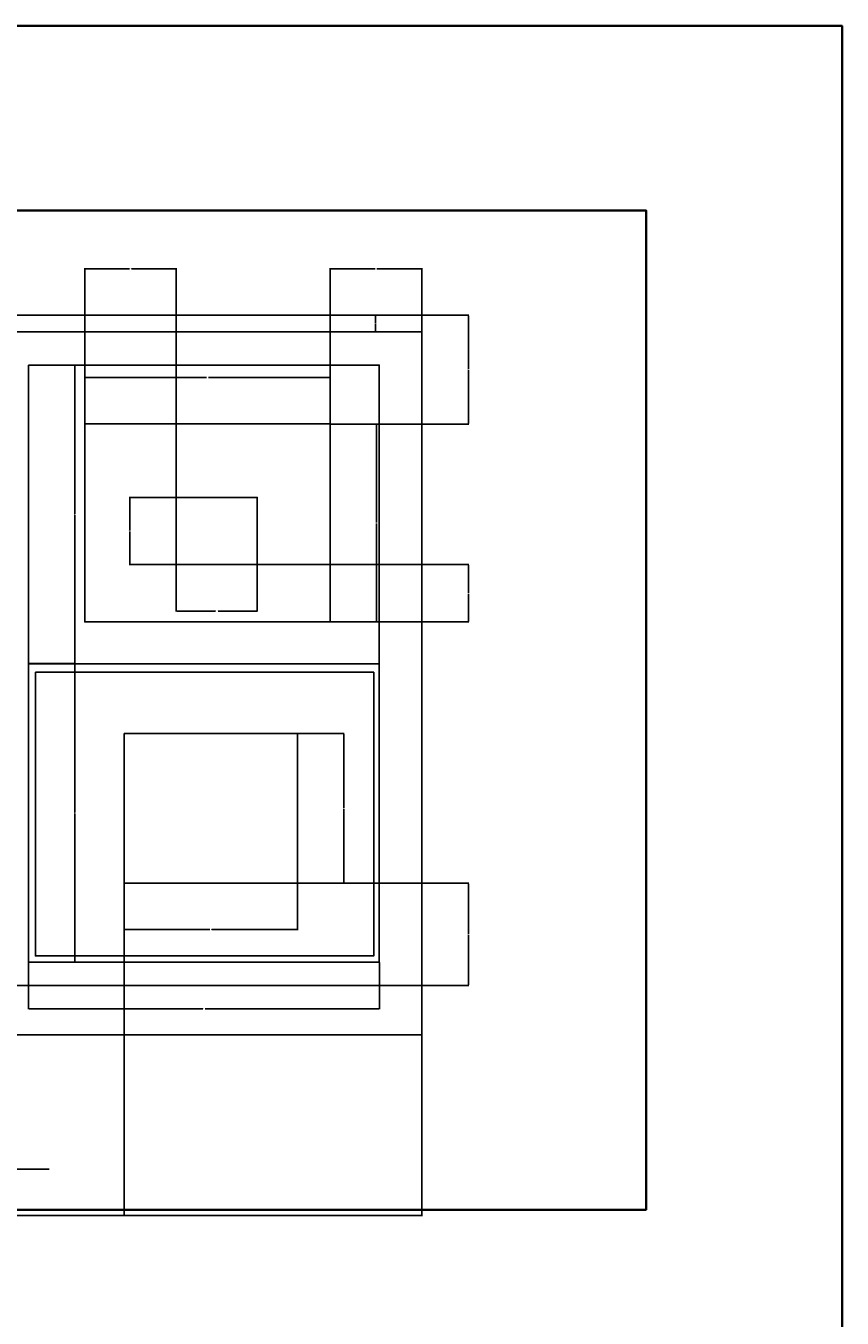
# Model space of a CAD drawing. Units: inches. Extents: x 1976 to 2558, y -977 to 2909.
# Tile 8 of 8: x 2262 to 2558, y 2441 to 2909. Entities that reach past the tile are written whole.
import ezdxf

# ---------------------------------------------------------------- set-up
doc = ezdxf.new("R2010")
doc.units = ezdxf.units.IN
for name, color, linetype, lineweight in [('A-ANNO-DIMS', 2, 'Continuous', 18), ('A-ANNO-TEXT', 7, 'Continuous', 25), ('A-ANNO-TTLB', 7, 'Continuous', 35), ('A-ELEV', 7, 'Continuous', 25)]:
    doc.layers.add(name, color=color, linetype=linetype, lineweight=lineweight)
doc.styles.get("Standard").update_dxf_attribs({"font": 'arial.ttf'})
doc.dimstyles.get("Standard").update_dxf_attribs({"dimtxt": 0.18, "dimasz": 0.18, "dimexe": 0.18, "dimexo": 0.0625, "dimgap": 0.09, "dimtad": 0, "dimtih": 1, "dimtoh": 1, "dimdec": 4, "dimzin": 0, "dimdsep": 46, "dimtxsty": 'Standard', "dimcen": 0.09, "dimadec": 0, "dimazin": 0, "dimtfac": 1, "dimtdec": 4, "dimtofl": 0, "dimtmove": 0, "dimatfit": 3, "dimfxl": 1, "dimtolj": 1, "dimtzin": 0, "dimarcsym": 0})

# ---------------------------------------------------------------- blocks, each defined once
blk = doc.blocks.new('*D51')
at = {"layer": 'A-ANNO-DIMS', "color": 0, "lineweight": -2, "transparency": 16777216}
for p, q in [((2089.7, 2681.2), (2089.7, 2477.53)), ((2405.44, 2543.2), (2405.44, 2477.53)), ((2089.88, 2477.71), (2247.1, 2477.71)), ((2405.26, 2477.71), (2248.03, 2477.71))]:
    blk.add_line(p, q, dxfattribs=at)
at = {"layer": 'A-ANNO-DIMS', "color": 0, "transparency": 16777216}
for points in [[(2089.88, 2477.74), (2089.88, 2477.68), (2089.7, 2477.71)], [(2405.26, 2477.74), (2405.26, 2477.68), (2405.44, 2477.71)]]:
    blk.add_solid(points, dxfattribs=at)
at = {"layer": 'Defpoints', "color": 0, "transparency": 16777216}
for p in [(2089.7, 2681.26), (2405.44, 2543.26), (2405.44, 2477.71)]:
    blk.add_point(p, dxfattribs=at)
at = {"layer": 'A-ANNO-DIMS', "color": 0, "transparency": 16777216, "insert": (2247.57, 2477.71), "char_height": 0.18, "attachment_point": 5}
blk.add_mtext('\\A1;315.74', dxfattribs=at)
blk = doc.blocks.new('*D63')
at = {"layer": 'A-ANNO-DIMS', "color": 0, "lineweight": -2, "transparency": 16777216}
for p, q in [((2372.2, 2764.9), (2389.17, 2764.9)), ((2388.99, 2764.72), (2388.99, 2729.2)), ((2388.99, 2693.31), (2388.99, 2728.83)), ((2372.2, 2693.13), (2389.17, 2693.13))]:
    blk.add_line(p, q, dxfattribs=at)
at = {"layer": 'A-ANNO-DIMS', "color": 0, "transparency": 16777216}
for points in [[(2388.96, 2764.72), (2389.02, 2764.72), (2388.99, 2764.9)], [(2388.96, 2693.31), (2389.02, 2693.31), (2388.99, 2693.13)]]:
    blk.add_solid(points, dxfattribs=at)
at = {"layer": 'Defpoints', "color": 0, "transparency": 16777216}
for p in [(2372.14, 2764.9), (2372.14, 2693.13), (2388.99, 2693.13)]:
    blk.add_point(p, dxfattribs=at)
at = {"layer": 'A-ANNO-DIMS', "color": 0, "transparency": 16777216, "insert": (2388.99, 2729.02), "char_height": 0.18, "attachment_point": 5}
blk.add_mtext('\\A1;71.77', dxfattribs=at)
blk = doc.blocks.new('*D64')
at = {"layer": 'A-ANNO-DIMS', "color": 0, "lineweight": -2, "transparency": 16777216}
for p, q in [((2283.12, 2764.97), (2283.12, 2781.93)), ((2283.3, 2781.75), (2327.23, 2781.75)), ((2371.96, 2781.75), (2328.02, 2781.75)), ((2372.14, 2764.97), (2372.14, 2781.93))]:
    blk.add_line(p, q, dxfattribs=at)
at = {"layer": 'A-ANNO-DIMS', "color": 0, "transparency": 16777216}
for points in [[(2283.3, 2781.78), (2283.3, 2781.72), (2283.12, 2781.75)], [(2371.96, 2781.78), (2371.96, 2781.72), (2372.14, 2781.75)]]:
    blk.add_solid(points, dxfattribs=at)
at = {"layer": 'Defpoints', "color": 0, "transparency": 16777216}
for p in [(2372.14, 2781.75), (2283.12, 2764.9), (2372.14, 2764.9)]:
    blk.add_point(p, dxfattribs=at)
at = {"layer": 'A-ANNO-DIMS', "color": 0, "transparency": 16777216, "insert": (2327.63, 2781.75), "char_height": 0.18, "attachment_point": 5}
blk.add_mtext('\\A1;89.02', dxfattribs=at)
blk = doc.blocks.new('*D65')
at = {"layer": 'A-ANNO-DIMS', "color": 0, "lineweight": -2, "transparency": 16777216}
for p, q in [((2297.4, 2598.25), (2297.4, 2581.28)), ((2360.24, 2598.25), (2360.24, 2581.28)), ((2297.58, 2581.46), (2328.43, 2581.46)), ((2360.06, 2581.46), (2329.21, 2581.46))]:
    blk.add_line(p, q, dxfattribs=at)
at = {"layer": 'A-ANNO-DIMS', "color": 0, "transparency": 16777216}
for points in [[(2297.58, 2581.49), (2297.58, 2581.43), (2297.4, 2581.46)], [(2360.06, 2581.49), (2360.06, 2581.43), (2360.24, 2581.46)]]:
    blk.add_solid(points, dxfattribs=at)
at = {"layer": 'Defpoints', "color": 0, "transparency": 16777216}
for p in [(2297.4, 2598.31), (2360.24, 2598.31), (2297.4, 2581.46)]:
    blk.add_point(p, dxfattribs=at)
at = {"layer": 'A-ANNO-DIMS', "color": 0, "transparency": 16777216, "insert": (2328.82, 2581.46), "char_height": 0.18, "attachment_point": 5}
blk.add_mtext('\\A1;62.84', dxfattribs=at)
blk = doc.blocks.new('*D66')
at = {"layer": 'A-ANNO-DIMS', "color": 0, "lineweight": -2, "transparency": 16777216}
for p, q in [((2360.3, 2652.57), (2377.27, 2652.57)), ((2377.09, 2652.39), (2377.09, 2625.62)), ((2377.09, 2598.49), (2377.09, 2625.26)), ((2360.3, 2598.31), (2377.27, 2598.31))]:
    blk.add_line(p, q, dxfattribs=at)
at = {"layer": 'A-ANNO-DIMS', "color": 0, "transparency": 16777216}
for points in [[(2377.06, 2652.39), (2377.12, 2652.39), (2377.09, 2652.57)], [(2377.06, 2598.49), (2377.12, 2598.49), (2377.09, 2598.31)]]:
    blk.add_solid(points, dxfattribs=at)
at = {"layer": 'Defpoints', "color": 0, "transparency": 16777216}
for p in [(2360.24, 2652.57), (2360.24, 2598.31), (2377.09, 2598.31)]:
    blk.add_point(p, dxfattribs=at)
at = {"layer": 'A-ANNO-DIMS', "color": 0, "transparency": 16777216, "insert": (2377.09, 2625.44), "char_height": 0.18, "attachment_point": 5}
blk.add_mtext('\\A1;54.26', dxfattribs=at)
blk = doc.blocks.new('*D67')
at = {"layer": 'A-ANNO-DIMS', "color": 0, "lineweight": -2, "transparency": 16777216}
for p, q in [((2297.4, 2598.25), (2297.4, 2477.53)), ((2249.44, 2561.2), (2249.44, 2477.53)), ((2249.62, 2477.71), (2273.02, 2477.71)), ((2297.22, 2477.71), (2273.82, 2477.71))]:
    blk.add_line(p, q, dxfattribs=at)
at = {"layer": 'A-ANNO-DIMS', "color": 0, "transparency": 16777216}
for points in [[(2249.62, 2477.74), (2249.62, 2477.68), (2249.44, 2477.71)], [(2297.22, 2477.74), (2297.22, 2477.68), (2297.4, 2477.71)]]:
    blk.add_solid(points, dxfattribs=at)
at = {"layer": 'Defpoints', "color": 0, "transparency": 16777216}
for p in [(2297.4, 2598.31), (2249.44, 2561.26), (2249.44, 2477.71)]:
    blk.add_point(p, dxfattribs=at)
at = {"layer": 'A-ANNO-DIMS', "color": 0, "transparency": 16777216, "insert": (2273.42, 2477.71), "char_height": 0.18, "attachment_point": 5}
blk.add_mtext('\\A1;47.96', dxfattribs=at)
blk = doc.blocks.new('*D68')
at = {"layer": 'A-ANNO-DIMS', "color": 0, "lineweight": -2, "transparency": 16777216}
for p, q in [((2372.14, 2764.97), (2372.14, 2821.39)), ((2372.32, 2821.21), (2388.46, 2821.21)), ((2405.26, 2821.21), (2389.11, 2821.21)), ((2405.44, 2804.43), (2405.44, 2821.39))]:
    blk.add_line(p, q, dxfattribs=at)
at = {"layer": 'A-ANNO-DIMS', "color": 0, "transparency": 16777216}
for points in [[(2372.32, 2821.24), (2372.32, 2821.18), (2372.14, 2821.21)], [(2405.26, 2821.24), (2405.26, 2821.18), (2405.44, 2821.21)]]:
    blk.add_solid(points, dxfattribs=at)
at = {"layer": 'Defpoints', "color": 0, "transparency": 16777216}
for p in [(2405.44, 2821.21), (2405.44, 2804.36), (2372.14, 2764.9)]:
    blk.add_point(p, dxfattribs=at)
at = {"layer": 'A-ANNO-DIMS', "color": 0, "transparency": 16777216, "insert": (2388.79, 2821.21), "char_height": 0.18, "attachment_point": 5}
blk.add_mtext('\\A1;33.3', dxfattribs=at)
blk = doc.blocks.new('*D69')
at = {"layer": 'A-ANNO-DIMS', "color": 0, "lineweight": -2, "transparency": 16777216}
for p, q in [((2405.5, 2804.36), (2422.47, 2804.36)), ((2422.29, 2804.18), (2422.29, 2784.81)), ((2422.29, 2765.08), (2422.29, 2784.45)), ((2372.2, 2764.9), (2422.47, 2764.9))]:
    blk.add_line(p, q, dxfattribs=at)
at = {"layer": 'A-ANNO-DIMS', "color": 0, "transparency": 16777216}
for points in [[(2422.26, 2804.18), (2422.32, 2804.18), (2422.29, 2804.36)], [(2422.26, 2765.08), (2422.32, 2765.08), (2422.29, 2764.9)]]:
    blk.add_solid(points, dxfattribs=at)
at = {"layer": 'Defpoints', "color": 0, "transparency": 16777216}
for p in [(2405.44, 2804.36), (2422.29, 2804.36), (2372.14, 2764.9)]:
    blk.add_point(p, dxfattribs=at)
at = {"layer": 'A-ANNO-DIMS', "color": 0, "transparency": 16777216, "insert": (2422.29, 2784.63), "char_height": 0.18, "attachment_point": 5}
blk.add_mtext('\\A1;39.46', dxfattribs=at)
blk = doc.blocks.new('*D70')
at = {"layer": 'A-ANNO-DIMS', "color": 0, "lineweight": -2, "transparency": 16777216}
for p, q in [((2360.3, 2598.31), (2422.47, 2598.31)), ((2422.29, 2598.13), (2422.29, 2579.97)), ((2422.29, 2561.44), (2422.29, 2579.6)), ((2405.5, 2561.26), (2422.47, 2561.26))]:
    blk.add_line(p, q, dxfattribs=at)
at = {"layer": 'A-ANNO-DIMS', "color": 0, "transparency": 16777216}
for points in [[(2422.26, 2598.13), (2422.32, 2598.13), (2422.29, 2598.31)], [(2422.26, 2561.44), (2422.32, 2561.44), (2422.29, 2561.26)]]:
    blk.add_solid(points, dxfattribs=at)
at = {"layer": 'Defpoints', "color": 0, "transparency": 16777216}
for p in [(2360.24, 2598.31), (2405.44, 2561.26), (2422.29, 2561.26)]:
    blk.add_point(p, dxfattribs=at)
at = {"layer": 'A-ANNO-DIMS', "color": 0, "transparency": 16777216, "insert": (2422.29, 2579.79), "char_height": 0.18, "attachment_point": 5}
blk.add_mtext('\\A1;37.05', dxfattribs=at)
blk = doc.blocks.new('*D80')
at = {"layer": 'A-ANNO-DIMS', "color": 0, "lineweight": -2, "transparency": 16777216}
for p, q in [((2316.29, 2713.84), (2316.29, 2696.87)), ((2345.68, 2713.84), (2345.68, 2696.87)), ((2316.47, 2697.05), (2330.52, 2697.05)), ((2345.5, 2697.05), (2331.45, 2697.05))]:
    blk.add_line(p, q, dxfattribs=at)
at = {"layer": 'A-ANNO-DIMS', "color": 0, "transparency": 16777216}
for points in [[(2316.47, 2697.08), (2316.47, 2697.02), (2316.29, 2697.05)], [(2345.5, 2697.08), (2345.5, 2697.02), (2345.68, 2697.05)]]:
    blk.add_solid(points, dxfattribs=at)
at = {"layer": 'Defpoints', "color": 0, "transparency": 16777216}
for p in [(2316.29, 2713.9), (2345.68, 2713.9), (2316.29, 2697.05)]:
    blk.add_point(p, dxfattribs=at)
at = {"layer": 'A-ANNO-DIMS', "color": 0, "transparency": 16777216, "insert": (2330.99, 2697.05), "char_height": 0.18, "attachment_point": 5}
blk.add_mtext('\\A1;29.394', dxfattribs=at)
blk = doc.blocks.new('*D81')
at = {"layer": 'A-ANNO-DIMS', "color": 0, "lineweight": -2, "transparency": 16777216}
for p, q in [((2316.23, 2738.25), (2299.26, 2738.25)), ((2299.44, 2738.07), (2299.44, 2726.26)), ((2299.44, 2714.08), (2299.44, 2725.9)), ((2316.23, 2713.9), (2299.26, 2713.9))]:
    blk.add_line(p, q, dxfattribs=at)
at = {"layer": 'A-ANNO-DIMS', "color": 0, "transparency": 16777216}
for points in [[(2299.41, 2738.07), (2299.47, 2738.07), (2299.44, 2738.25)], [(2299.41, 2714.08), (2299.47, 2714.08), (2299.44, 2713.9)]]:
    blk.add_solid(points, dxfattribs=at)
at = {"layer": 'Defpoints', "color": 0, "transparency": 16777216}
for p in [(2299.44, 2738.25), (2316.29, 2738.25), (2316.29, 2713.9)]:
    blk.add_point(p, dxfattribs=at)
at = {"layer": 'A-ANNO-DIMS', "color": 0, "transparency": 16777216, "insert": (2299.44, 2726.08), "char_height": 0.18, "attachment_point": 5}
blk.add_mtext('\\A1;24.345', dxfattribs=at)
blk = doc.blocks.new('*D82')
at = {"layer": 'A-ANNO-DIMS', "color": 0, "lineweight": -2, "transparency": 16777216}
for p, q in [((2405.38, 2804.36), (2388.41, 2804.36)), ((2388.59, 2804.18), (2388.59, 2801.54)), ((2388.59, 2798.54), (2388.59, 2801.18)), ((2405.38, 2798.36), (2388.41, 2798.36))]:
    blk.add_line(p, q, dxfattribs=at)
at = {"layer": 'A-ANNO-DIMS', "color": 0, "transparency": 16777216}
for points in [[(2388.56, 2804.18), (2388.62, 2804.18), (2388.59, 2804.36)], [(2388.56, 2798.54), (2388.62, 2798.54), (2388.59, 2798.36)]]:
    blk.add_solid(points, dxfattribs=at)
at = {"layer": 'Defpoints', "color": 0, "transparency": 16777216}
for p in [(2388.59, 2804.36), (2405.44, 2804.36), (2405.44, 2798.36)]:
    blk.add_point(p, dxfattribs=at)
at = {"layer": 'A-ANNO-DIMS', "color": 0, "transparency": 16777216, "insert": (2388.59, 2801.36), "char_height": 0.18, "attachment_point": 5}
blk.add_mtext('\\A1;6', dxfattribs=at)
blk = doc.blocks.new('*D83')
at = {"layer": 'A-ANNO-DIMS', "color": 0, "lineweight": -2, "transparency": 16777216}
for p, q in [((2283.12, 2764.97), (2283.12, 2821.39)), ((2283.3, 2821.21), (2299.31, 2821.21)), ((2316.11, 2821.21), (2300.1, 2821.21)), ((2316.29, 2738.31), (2316.29, 2821.39))]:
    blk.add_line(p, q, dxfattribs=at)
at = {"layer": 'A-ANNO-DIMS', "color": 0, "transparency": 16777216}
for points in [[(2283.3, 2821.24), (2283.3, 2821.18), (2283.12, 2821.21)], [(2316.11, 2821.24), (2316.11, 2821.18), (2316.29, 2821.21)]]:
    blk.add_solid(points, dxfattribs=at)
at = {"layer": 'Defpoints', "color": 0, "transparency": 16777216}
for p in [(2283.12, 2821.21), (2283.12, 2764.9), (2316.29, 2738.25)]:
    blk.add_point(p, dxfattribs=at)
at = {"layer": 'A-ANNO-DIMS', "color": 0, "transparency": 16777216, "insert": (2299.7, 2821.21), "char_height": 0.18, "attachment_point": 5}
blk.add_mtext('\\A1;33.17', dxfattribs=at)
blk = doc.blocks.new('*D84')
at = {"layer": 'A-ANNO-DIMS', "color": 0, "lineweight": -2, "transparency": 16777216}
for p, q in [((2345.74, 2713.9), (2422.47, 2713.9)), ((2422.29, 2713.72), (2422.29, 2703.7)), ((2422.29, 2693.31), (2422.29, 2703.33)), ((2372.2, 2693.13), (2422.47, 2693.13))]:
    blk.add_line(p, q, dxfattribs=at)
at = {"layer": 'A-ANNO-DIMS', "color": 0, "transparency": 16777216}
for points in [[(2422.26, 2713.72), (2422.32, 2713.72), (2422.29, 2713.9)], [(2422.26, 2693.31), (2422.32, 2693.31), (2422.29, 2693.13)]]:
    blk.add_solid(points, dxfattribs=at)
at = {"layer": 'Defpoints', "color": 0, "transparency": 16777216}
for p in [(2345.68, 2713.9), (2372.14, 2693.13), (2422.29, 2693.13)]:
    blk.add_point(p, dxfattribs=at)
at = {"layer": 'A-ANNO-DIMS', "color": 0, "transparency": 16777216, "insert": (2422.29, 2703.52), "char_height": 0.18, "attachment_point": 5}
blk.add_mtext('\\A1;20.777', dxfattribs=at)
blk = doc.blocks.new('*D85')
at = {"layer": 'A-ANNO-DIMS', "color": 0, "lineweight": -2, "transparency": 16777216}
for p, q in [((2262.7, 2569.55), (2262.7, 2552.58)), ((2389.98, 2569.55), (2389.98, 2552.58)), ((2262.88, 2552.76), (2325.89, 2552.76)), ((2389.8, 2552.76), (2326.8, 2552.76))]:
    blk.add_line(p, q, dxfattribs=at)
at = {"layer": 'A-ANNO-DIMS', "color": 0, "transparency": 16777216}
for points in [[(2262.88, 2552.79), (2262.88, 2552.73), (2262.7, 2552.76)], [(2389.8, 2552.79), (2389.8, 2552.73), (2389.98, 2552.76)]]:
    blk.add_solid(points, dxfattribs=at)
at = {"layer": 'Defpoints', "color": 0, "transparency": 16777216}
for p in [(2262.7, 2569.61), (2389.98, 2569.61), (2262.7, 2552.76)]:
    blk.add_point(p, dxfattribs=at)
at = {"layer": 'A-ANNO-DIMS', "color": 0, "transparency": 16777216, "insert": (2326.34, 2552.76), "char_height": 0.18, "attachment_point": 5}
blk.add_mtext('\\A1;127.27', dxfattribs=at)
blk = doc.blocks.new('*D86')
at = {"layer": 'A-ANNO-DIMS', "color": 0, "lineweight": -2, "transparency": 16777216}
for p, q in [((2262.77, 2786.3), (2279.73, 2786.3)), ((2279.55, 2786.12), (2279.55, 2732.31)), ((2279.55, 2678.14), (2279.55, 2731.95)), ((2262.77, 2677.96), (2279.73, 2677.96))]:
    blk.add_line(p, q, dxfattribs=at)
at = {"layer": 'A-ANNO-DIMS', "color": 0, "transparency": 16777216}
for points in [[(2279.52, 2786.12), (2279.58, 2786.12), (2279.55, 2786.3)], [(2279.52, 2678.14), (2279.58, 2678.14), (2279.55, 2677.96)]]:
    blk.add_solid(points, dxfattribs=at)
at = {"layer": 'Defpoints', "color": 0, "transparency": 16777216}
for p in [(2262.7, 2786.3), (2262.7, 2677.96), (2279.55, 2677.96)]:
    blk.add_point(p, dxfattribs=at)
at = {"layer": 'A-ANNO-DIMS', "color": 0, "transparency": 16777216, "insert": (2279.55, 2732.13), "char_height": 0.18, "attachment_point": 5}
blk.add_mtext('\\A1;108.35', dxfattribs=at)
blk = doc.blocks.new('*D87')
at = {"layer": 'A-ANNO-DIMS', "color": 0, "lineweight": -2, "transparency": 16777216}
for p, q in [((2262.77, 2677.96), (2279.73, 2677.96)), ((2279.55, 2677.78), (2279.55, 2623.96)), ((2279.55, 2569.79), (2279.55, 2623.6)), ((2262.77, 2569.61), (2279.73, 2569.61))]:
    blk.add_line(p, q, dxfattribs=at)
at = {"layer": 'A-ANNO-DIMS', "color": 0, "transparency": 16777216}
for points in [[(2279.52, 2677.78), (2279.58, 2677.78), (2279.55, 2677.96)], [(2279.52, 2569.79), (2279.58, 2569.79), (2279.55, 2569.61)]]:
    blk.add_solid(points, dxfattribs=at)
at = {"layer": 'Defpoints', "color": 0, "transparency": 16777216}
for p in [(2262.7, 2677.96), (2262.7, 2569.61), (2279.55, 2569.61)]:
    blk.add_point(p, dxfattribs=at)
at = {"layer": 'A-ANNO-DIMS', "color": 0, "transparency": 16777216, "insert": (2279.55, 2623.78), "char_height": 0.18, "attachment_point": 5}
blk.add_mtext('\\A1;108.35', dxfattribs=at)

msp = doc.modelspace()

# ---------------------------------------------------------------- linework, layer by layer
at = {"layer": 'A-ANNO-TEXT'}
msp.add_line((2175.0551, 2494.5563), (2270.2236, 2494.5563), dxfattribs=at)
at = {"layer": 'A-ANNO-TTLB'}
for points in [[(1975.8545, 2909.3429), (2557.9168, 2909.3429), (2557.9168, 1747.8598), (1975.8545, 1747.8598)], [(2026.154, 2842.3802), (2486.7724, 2842.3802), (2486.7724, 2479.8768), (2026.154, 2479.8768)]]:
    msp.add_lwpolyline(points, close=True, dxfattribs=at)
at = {"layer": 'A-ELEV'}
for p, q in [((2405.4385, 2804.3628), (2242.2431, 2804.3628)), ((2405.4385, 2729.2601), (2405.4385, 2804.3628)), ((2242.2431, 2798.3628), (2405.4385, 2798.3628)), ((2405.4385, 2729.2601), (2405.4385, 2543.2601)), ((2262.7036, 2677.9562), (2389.9779, 2677.9562)), ((2405.4385, 2561.2601), (2108.4385, 2561.2601)), ((2405.4385, 2543.2601), (2108.4385, 2543.2601))]:
    msp.add_line(p, q, dxfattribs=at)
for points in [[(2262.7036, 2786.3045), (2389.9779, 2786.3045), (2389.9779, 2569.6078), (2262.7036, 2569.6078)], [(2283.1154, 2764.9027), (2372.1361, 2764.9027), (2372.1361, 2693.1279), (2283.1154, 2693.1279)], [(2316.2882, 2738.2495), (2345.6818, 2738.2495), (2345.6818, 2713.9048), (2316.2882, 2713.9048)], [(2265.2047, 2674.8279), (2387.968, 2674.8279), (2387.968, 2571.9459), (2265.2047, 2571.9459)], [(2297.4015, 2652.5694), (2360.2409, 2652.5694), (2360.2409, 2598.3119), (2297.4015, 2598.3119)]]:
    msp.add_lwpolyline(points, close=True, dxfattribs=at)

# ---------------------------------------------------------------- dimensions: what is measured, and where the dimension line sits
at = {"layer": 'A-ANNO-DIMS'}
for base, p1, p2, override, picture, middle in [((2283.1154, 2821.2128), (2316.2882, 2738.2495), (2283.1154, 2764.9027), {"dimdec": 2, "dimlfac": 1, "dimrnd": 0, "dimzin": 0, "dimdsep": 46, "dimlunit": 2}, '*D83', (2299.7018, 2821.2128)), ((2405.4385, 2821.2128), (2372.1361, 2764.9027), (2405.4385, 2804.3628), {"dimdec": 1, "dimlfac": 1, "dimrnd": 0, "dimzin": 0, "dimdsep": 46, "dimlunit": 2}, '*D68', (2388.7873, 2821.2128)), ((2372.1361, 2781.7527), (2283.1154, 2764.9027), (2372.1361, 2764.9027), {"dimdec": 2, "dimlfac": 1, "dimrnd": 0, "dimzin": 0, "dimdsep": 46, "dimlunit": 2}, '*D64', (2327.6258, 2781.7527)), ((2405.4385, 2477.7063), (2089.697, 2681.2601), (2405.4385, 2543.2601), {"dimdec": 2, "dimlfac": 1, "dimrnd": 0, "dimzin": 0, "dimdsep": 46, "dimlunit": 2}, '*D51', (2247.5677, 2477.7063)), ((2249.4385, 2477.7063), (2297.4015, 2598.3119), (2249.4385, 2561.2601), {"dimdec": 2, "dimlfac": 1, "dimrnd": 0, "dimzin": 0, "dimdsep": 46, "dimlunit": 2}, '*D67', (2273.42, 2477.7063))]:
    dim = msp.add_linear_dim(base=base, p1=p1, p2=p2, dimstyle='Standard', override=override, dxfattribs=at)
    dim.commit()
    dim.dimension.update_dxf_attribs({"geometry": picture, "text_midpoint": middle})
for base, p1, p2, angle, override, picture, middle in [((2422.2885, 2804.3628), (2372.1361, 2764.9027), (2405.4385, 2804.3628), 90, {"dimdec": 2, "dimlfac": 1, "dimrnd": 0, "dimzin": 0, "dimdsep": 46, "dimlunit": 2}, '*D69', (2422.2885, 2784.6327)), ((2388.5885, 2804.3628), (2405.4385, 2798.3628), (2405.4385, 2804.3628), 90, {"dimdec": 0, "dimlfac": 1, "dimrnd": 0, "dimzin": 0, "dimdsep": 46, "dimlunit": 2}, '*D82', (2388.5885, 2801.3628)), ((2279.5536, 2677.9562), (2262.7036, 2786.3045), (2262.7036, 2677.9562), 270, {"dimdec": 2, "dimlfac": 1, "dimrnd": 0, "dimzin": 0, "dimdsep": 46, "dimlunit": 2}, '*D86', (2279.5536, 2732.1303)), ((2388.9861, 2693.1279), (2372.1361, 2764.9027), (2372.1361, 2693.1279), 270, {"dimdec": 2, "dimlfac": 1, "dimrnd": 0, "dimzin": 0, "dimdsep": 46, "dimlunit": 2}, '*D63', (2388.9861, 2729.0153)), ((2299.4382, 2738.2495), (2316.2882, 2713.9048), (2316.2882, 2738.2495), 90, {"dimdec": 3, "dimlfac": 1, "dimrnd": 0, "dimzin": 0, "dimdsep": 46, "dimlunit": 2}, '*D81', (2299.4382, 2726.0771)), ((2316.2882, 2697.0548), (2345.6818, 2713.9048), (2316.2882, 2713.9048), 180, {"dimdec": 3, "dimlfac": 1, "dimrnd": 0, "dimzin": 0, "dimdsep": 46, "dimlunit": 2}, '*D80', (2330.985, 2697.0548)), ((2422.2885, 2693.1279), (2345.6818, 2713.9048), (2372.1361, 2693.1279), 90, {"dimdec": 3, "dimlfac": 1, "dimrnd": 0, "dimzin": 0, "dimdsep": 46, "dimlunit": 2}, '*D84', (2422.2885, 2703.5163)), ((2279.5536, 2569.6078), (2262.7036, 2677.9562), (2262.7036, 2569.6078), 270, {"dimdec": 2, "dimlfac": 1, "dimrnd": 0, "dimzin": 0, "dimdsep": 46, "dimlunit": 2}, '*D87', (2279.5536, 2623.782)), ((2377.0909, 2598.3119), (2360.2409, 2652.5694), (2360.2409, 2598.3119), 270, {"dimdec": 2, "dimlfac": 1, "dimrnd": 0, "dimzin": 0, "dimdsep": 46, "dimlunit": 2}, '*D66', (2377.0909, 2625.4407)), ((2297.4015, 2581.4619), (2360.2409, 2598.3119), (2297.4015, 2598.3119), 180, {"dimdec": 2, "dimlfac": 1, "dimrnd": 0, "dimzin": 0, "dimdsep": 46, "dimlunit": 2}, '*D65', (2328.8212, 2581.4619)), ((2422.2885, 2561.2601), (2360.2409, 2598.3119), (2405.4385, 2561.2601), 90, {"dimdec": 2, "dimlfac": 1, "dimrnd": 0, "dimzin": 0, "dimdsep": 46, "dimlunit": 2}, '*D70', (2422.2885, 2579.786)), ((2262.7036, 2552.7578), (2389.9779, 2569.6078), (2262.7036, 2569.6078), 180, {"dimdec": 2, "dimlfac": 1, "dimrnd": 0, "dimzin": 0, "dimdsep": 46, "dimlunit": 2}, '*D85', (2326.3408, 2552.7578))]:
    dim = msp.add_linear_dim(base=base, p1=p1, p2=p2, angle=angle, dimstyle='Standard', override=override, dxfattribs=at)
    dim.commit()
    dim.dimension.update_dxf_attribs({"geometry": picture, "text_midpoint": middle})

doc.saveas('drawing.dxf')
